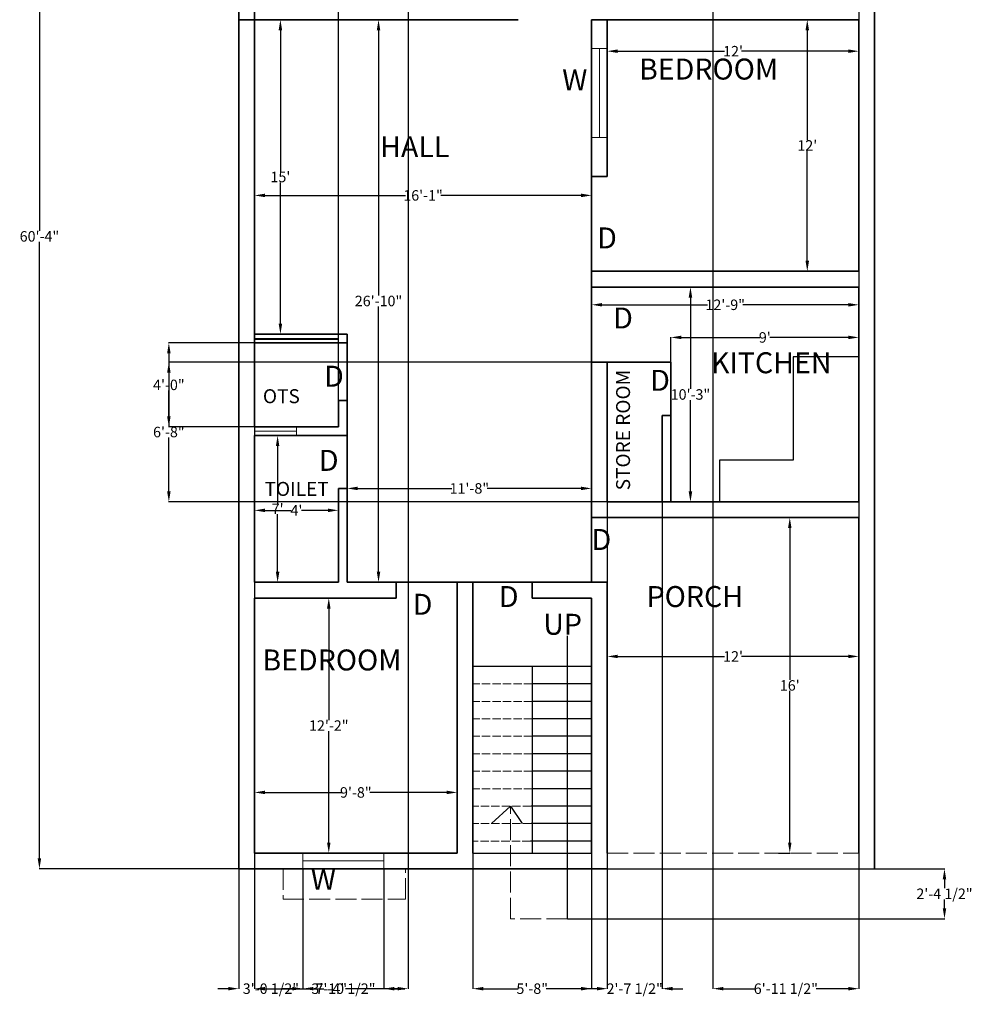
# Model space of a CAD drawing. Units: inches. Extents: x -732 to -187, y 754 to 1605.
# Tile 1 of 2: x -732 to -187, y 754 to 1318. Entities that reach past the tile are written whole.
import ezdxf

# ---------------------------------------------------------------- set-up
doc = ezdxf.new("R2010")
doc.units = ezdxf.units.IN
doc.header["$MEASUREMENT"] = 0
doc.linetypes.add('ACAD_ISO02W100', pattern=[15, 12, -3])
for name, color, linetype, lineweight in [('A-ANNO-DIMS', 2, 'Continuous', 18), ('A-ANNO-TEXT', 3, 'Continuous', 18), ('A-AREA-IDEN', 7, 'Continuous', 25), ('A-FLOR-CASE', 8, 'Continuous', 25), ('A-FLOR-STRS', 3, 'Continuous', 25), ('A-FLOR-STRS-HIDN', 3, 'ACAD_ISO02W100', 18), ('A-GLAZ', 4, 'Continuous', 18), ('A-ROOF-OVHD', 8, 'ACAD_ISO02W100', 18), ('A-WALL', 7, 'Continuous', 35)]:
    doc.layers.add(name, color=color, linetype=linetype, lineweight=lineweight)
doc.styles.get("Standard").update_dxf_attribs({"font": 'arial.ttf'})
doc.dimstyles.get("Standard").update_dxf_attribs({"dimtxt": 6, "dimasz": 6, "dimexe": 0.18, "dimexo": 0.0625, "dimgap": 0.09, "dimtad": 0, "dimtih": 1, "dimtoh": 1, "dimdec": 0, "dimzin": 0, "dimdsep": 46, "dimlunit": 3, "dimtxsty": 'Standard', "dimcen": 0.09, "dimadec": 0, "dimazin": 0, "dimtfac": 1, "dimtdec": 0, "dimtofl": 0, "dimtmove": 0, "dimatfit": 3, "dimfxl": 1, "dimtolj": 1, "dimtzin": 0, "dimarcsym": 0})

# ---------------------------------------------------------------- blocks, each defined once
blk = doc.blocks.new('*D4')
at = {"layer": 'A-ANNO-DIMS', "color": 0, "lineweight": -2, "transparency": 16777216}
for p, q in [((-597.28, 886.17), (-597.28, 875.44)), ((-481.28, 886.17), (-481.28, 875.44)), ((-591.28, 875.62), (-547.34, 875.62)), ((-487.28, 875.62), (-531.21, 875.62))]:
    blk.add_line(p, q, dxfattribs=at)
at = {"layer": 'A-ANNO-DIMS', "color": 0, "transparency": 16777216}
for points in [[(-591.28, 876.62), (-591.28, 874.62), (-597.28, 875.62)], [(-487.28, 876.62), (-487.28, 874.62), (-481.28, 875.62)]]:
    blk.add_solid(points, dxfattribs=at)
at = {"layer": 'Defpoints', "color": 0, "transparency": 16777216}
for p in [(-597.28, 886.23), (-481.28, 886.23), (-481.28, 875.62)]:
    blk.add_point(p, dxfattribs=at)
at = {"layer": 'A-ANNO-DIMS', "color": 0, "transparency": 16777216, "insert": (-539.28, 875.62), "char_height": 6, "attachment_point": 5}
blk.add_mtext('\\A1;9\'-8"', dxfattribs=at)
blk = doc.blocks.new('*D5')
at = {"layer": 'A-ANNO-DIMS', "color": 0, "lineweight": -2, "transparency": 16777216}
for p, q in [((-544.34, 986.88), (-554.94, 986.88)), ((-554.76, 980.88), (-554.76, 916.98)), ((-554.76, 846.88), (-554.76, 910.77)), ((-544.34, 840.88), (-554.94, 840.88))]:
    blk.add_line(p, q, dxfattribs=at)
at = {"layer": 'A-ANNO-DIMS', "color": 0, "transparency": 16777216}
for points in [[(-555.76, 980.88), (-553.76, 980.88), (-554.76, 986.88)], [(-555.76, 846.88), (-553.76, 846.88), (-554.76, 840.88)]]:
    blk.add_solid(points, dxfattribs=at)
at = {"layer": 'Defpoints', "color": 0, "transparency": 16777216}
for p in [(-544.28, 986.88), (-554.76, 840.88), (-544.28, 840.88)]:
    blk.add_point(p, dxfattribs=at)
at = {"layer": 'A-ANNO-DIMS', "color": 0, "transparency": 16777216, "insert": (-554.76, 913.88), "char_height": 6, "attachment_point": 5}
blk.add_mtext('\\A1;12\'-2"', dxfattribs=at)
blk = doc.blocks.new('*D6')
at = {"layer": 'A-ANNO-DIMS', "color": 0, "lineweight": -2, "transparency": 16777216}
for p, q in [((-297.29, 1032.88), (-290.63, 1032.88)), ((-290.81, 1026.88), (-290.81, 940.03)), ((-290.81, 846.88), (-290.81, 933.72)), ((-297.29, 840.88), (-290.63, 840.88))]:
    blk.add_line(p, q, dxfattribs=at)
at = {"layer": 'A-ANNO-DIMS', "color": 0, "transparency": 16777216}
for points in [[(-291.81, 1026.88), (-289.81, 1026.88), (-290.81, 1032.88)], [(-291.81, 846.88), (-289.81, 846.88), (-290.81, 840.88)]]:
    blk.add_solid(points, dxfattribs=at)
at = {"layer": 'Defpoints', "color": 0, "transparency": 16777216}
for p in [(-297.35, 1032.88), (-297.35, 840.88), (-290.81, 840.88)]:
    blk.add_point(p, dxfattribs=at)
at = {"layer": 'A-ANNO-DIMS', "color": 0, "transparency": 16777216, "insert": (-290.81, 936.88), "char_height": 6, "attachment_point": 5}
blk.add_mtext("\\A1;16'", dxfattribs=at)
blk = doc.blocks.new('*D7')
at = {"layer": 'A-ANNO-DIMS', "color": 0, "lineweight": -2, "transparency": 16777216}
for p, q in [((-395.28, 939.28), (-395.28, 953.64)), ((-389.28, 953.46), (-328.18, 953.46)), ((-257.28, 953.46), (-318.38, 953.46)), ((-251.28, 939.28), (-251.28, 953.64))]:
    blk.add_line(p, q, dxfattribs=at)
at = {"layer": 'A-ANNO-DIMS', "color": 0, "transparency": 16777216}
for points in [[(-389.28, 954.46), (-389.28, 952.46), (-395.28, 953.46)], [(-257.28, 954.46), (-257.28, 952.46), (-251.28, 953.46)]]:
    blk.add_solid(points, dxfattribs=at)
at = {"layer": 'Defpoints', "color": 0, "transparency": 16777216}
for p in [(-251.28, 953.46), (-395.28, 939.22), (-251.28, 939.22)]:
    blk.add_point(p, dxfattribs=at)
at = {"layer": 'A-ANNO-DIMS', "color": 0, "transparency": 16777216, "insert": (-323.28, 953.46), "char_height": 6, "attachment_point": 5}
blk.add_mtext("\\A1;12'", dxfattribs=at)
blk = doc.blocks.new('*D8')
at = {"layer": 'A-ANNO-DIMS', "color": 0, "lineweight": -2, "transparency": 16777216}
for p, q in [((-597.28, 1037.81), (-597.28, 1036.88)), ((-591.28, 1037.06), (-576.25, 1037.06)), ((-555.28, 1037.06), (-570.31, 1037.06)), ((-549.28, 1037.81), (-549.28, 1036.88))]:
    blk.add_line(p, q, dxfattribs=at)
at = {"layer": 'A-ANNO-DIMS', "color": 0, "transparency": 16777216}
for points in [[(-591.28, 1038.06), (-591.28, 1036.06), (-597.28, 1037.06)], [(-555.28, 1038.06), (-555.28, 1036.06), (-549.28, 1037.06)]]:
    blk.add_solid(points, dxfattribs=at)
at = {"layer": 'Defpoints', "color": 0, "transparency": 16777216}
for p in [(-597.28, 1037.88), (-549.28, 1037.88), (-549.28, 1037.06)]:
    blk.add_point(p, dxfattribs=at)
at = {"layer": 'A-ANNO-DIMS', "color": 0, "transparency": 16777216, "insert": (-573.28, 1037.06), "char_height": 6, "attachment_point": 5}
blk.add_mtext("\\A1;4'", dxfattribs=at)
blk = doc.blocks.new('*D9')
at = {"layer": 'A-ANNO-DIMS', "color": 0, "lineweight": -2, "transparency": 16777216}
for p, q in [((-587.22, 1079.88), (-583.88, 1079.88)), ((-584.06, 1073.88), (-584.06, 1040.97)), ((-584.06, 1001.88), (-584.06, 1034.79)), ((-587.22, 995.88), (-583.88, 995.88))]:
    blk.add_line(p, q, dxfattribs=at)
at = {"layer": 'A-ANNO-DIMS', "color": 0, "transparency": 16777216}
for points in [[(-585.06, 1073.88), (-583.06, 1073.88), (-584.06, 1079.88)], [(-585.06, 1001.88), (-583.06, 1001.88), (-584.06, 995.88)]]:
    blk.add_solid(points, dxfattribs=at)
at = {"layer": 'Defpoints', "color": 0, "transparency": 16777216}
for p in [(-587.28, 1079.88), (-587.28, 995.88), (-584.06, 995.88)]:
    blk.add_point(p, dxfattribs=at)
at = {"layer": 'A-ANNO-DIMS', "color": 0, "transparency": 16777216, "insert": (-584.06, 1037.88), "char_height": 6, "attachment_point": 5}
blk.add_mtext("\\A1;7'", dxfattribs=at)
blk = doc.blocks.new('*D10')
at = {"layer": 'A-ANNO-DIMS', "color": 0, "lineweight": -2, "transparency": 16777216}
for p, q in [((-544.28, 1049.68), (-544.28, 1049.8)), ((-538.28, 1049.62), (-484.39, 1049.62)), ((-410.28, 1049.62), (-464.17, 1049.62)), ((-404.28, 1049.68), (-404.28, 1049.8))]:
    blk.add_line(p, q, dxfattribs=at)
at = {"layer": 'A-ANNO-DIMS', "color": 0, "transparency": 16777216}
for points in [[(-538.28, 1050.62), (-538.28, 1048.62), (-544.28, 1049.62)], [(-410.28, 1050.62), (-410.28, 1048.62), (-404.28, 1049.62)]]:
    blk.add_solid(points, dxfattribs=at)
at = {"layer": 'Defpoints', "color": 0, "transparency": 16777216}
for p in [(-544.28, 1049.62), (-404.28, 1049.62), (-404.28, 1049.62)]:
    blk.add_point(p, dxfattribs=at)
at = {"layer": 'A-ANNO-DIMS', "color": 0, "transparency": 16777216, "insert": (-474.28, 1049.62), "char_height": 6, "attachment_point": 5}
blk.add_mtext('\\A1;11\'-8"', dxfattribs=at)
blk = doc.blocks.new('*D11')
at = {"layer": 'A-ANNO-DIMS', "color": 0, "lineweight": -2, "transparency": 16777216}
for p, q in [((-404.28, 1154.77), (-404.28, 1154.89)), ((-398.28, 1154.71), (-337.89, 1154.71)), ((-257.28, 1154.71), (-317.67, 1154.71)), ((-251.28, 1154.77), (-251.28, 1154.89))]:
    blk.add_line(p, q, dxfattribs=at)
at = {"layer": 'A-ANNO-DIMS', "color": 0, "transparency": 16777216}
for points in [[(-398.28, 1155.71), (-398.28, 1153.71), (-404.28, 1154.71)], [(-257.28, 1155.71), (-257.28, 1153.71), (-251.28, 1154.71)]]:
    blk.add_solid(points, dxfattribs=at)
at = {"layer": 'Defpoints', "color": 0, "transparency": 16777216}
for p in [(-404.28, 1154.71), (-251.28, 1154.71), (-251.28, 1154.71)]:
    blk.add_point(p, dxfattribs=at)
at = {"layer": 'A-ANNO-DIMS', "color": 0, "transparency": 16777216, "insert": (-327.78, 1154.71), "char_height": 6, "attachment_point": 5}
blk.add_mtext('\\A1;12\'-9"', dxfattribs=at)
blk = doc.blocks.new('*D12')
at = {"layer": 'A-ANNO-DIMS', "color": 0, "lineweight": -2, "transparency": 16777216}
for p, q in [((-347.74, 1164.88), (-347.86, 1164.88)), ((-347.68, 1158.88), (-347.68, 1106.53)), ((-347.68, 1047.88), (-347.68, 1100.22)), ((-347.74, 1041.88), (-347.86, 1041.88))]:
    blk.add_line(p, q, dxfattribs=at)
at = {"layer": 'A-ANNO-DIMS', "color": 0, "transparency": 16777216}
for points in [[(-348.68, 1158.88), (-346.68, 1158.88), (-347.68, 1164.88)], [(-348.68, 1047.88), (-346.68, 1047.88), (-347.68, 1041.88)]]:
    blk.add_solid(points, dxfattribs=at)
at = {"layer": 'Defpoints', "color": 0, "transparency": 16777216}
for p in [(-347.68, 1164.88), (-347.68, 1041.88), (-347.68, 1041.88)]:
    blk.add_point(p, dxfattribs=at)
at = {"layer": 'A-ANNO-DIMS', "color": 0, "transparency": 16777216, "insert": (-347.68, 1103.38), "char_height": 6, "attachment_point": 5}
blk.add_mtext('\\A1;10\'-3"', dxfattribs=at)
blk = doc.blocks.new('*D13')
at = {"layer": 'A-ANNO-DIMS', "color": 0, "lineweight": -2, "transparency": 16777216}
for p, q in [((-358.95, 1121.95), (-358.95, 1136.21)), ((-352.95, 1136.03), (-307.96, 1136.03)), ((-257.28, 1136.03), (-302.26, 1136.03)), ((-251.28, 1125.07), (-251.28, 1136.21))]:
    blk.add_line(p, q, dxfattribs=at)
at = {"layer": 'A-ANNO-DIMS', "color": 0, "transparency": 16777216}
for points in [[(-352.95, 1137.03), (-352.95, 1135.03), (-358.95, 1136.03)], [(-257.28, 1137.03), (-257.28, 1135.03), (-251.28, 1136.03)]]:
    blk.add_solid(points, dxfattribs=at)
at = {"layer": 'Defpoints', "color": 0, "transparency": 16777216}
for p in [(-251.28, 1136.03), (-358.95, 1121.89), (-251.28, 1125.01)]:
    blk.add_point(p, dxfattribs=at)
at = {"layer": 'A-ANNO-DIMS', "color": 0, "transparency": 16777216, "insert": (-305.11, 1136.03), "char_height": 6, "attachment_point": 5}
blk.add_mtext("\\A1;9'", dxfattribs=at)
blk = doc.blocks.new('*D14')
at = {"layer": 'A-ANNO-DIMS', "color": 0, "lineweight": -2, "transparency": 16777216}
for p, q in [((-585.31, 1317.88), (-582.28, 1317.88)), ((-582.46, 1311.88), (-582.46, 1231.03)), ((-582.46, 1143.88), (-582.46, 1224.72)), ((-585.31, 1137.88), (-582.28, 1137.88))]:
    blk.add_line(p, q, dxfattribs=at)
at = {"layer": 'A-ANNO-DIMS', "color": 0, "transparency": 16777216}
for points in [[(-583.46, 1311.88), (-581.46, 1311.88), (-582.46, 1317.88)], [(-583.46, 1143.88), (-581.46, 1143.88), (-582.46, 1137.88)]]:
    blk.add_solid(points, dxfattribs=at)
at = {"layer": 'Defpoints', "color": 0, "transparency": 16777216}
for p in [(-585.37, 1317.88), (-585.37, 1137.88), (-582.46, 1137.88)]:
    blk.add_point(p, dxfattribs=at)
at = {"layer": 'A-ANNO-DIMS', "color": 0, "transparency": 16777216, "insert": (-582.46, 1227.88), "char_height": 6, "attachment_point": 5}
blk.add_mtext("\\A1;15'", dxfattribs=at)
blk = doc.blocks.new('*D15')
at = {"layer": 'A-ANNO-DIMS', "color": 0, "lineweight": -2, "transparency": 16777216}
for p, q in [((-251.34, 1317.88), (-280.96, 1317.88)), ((-280.78, 1311.88), (-280.78, 1248.98)), ((-280.78, 1179.88), (-280.78, 1242.77)), ((-251.34, 1173.88), (-280.96, 1173.88))]:
    blk.add_line(p, q, dxfattribs=at)
at = {"layer": 'A-ANNO-DIMS', "color": 0, "transparency": 16777216}
for points in [[(-281.78, 1311.88), (-279.78, 1311.88), (-280.78, 1317.88)], [(-281.78, 1179.88), (-279.78, 1179.88), (-280.78, 1173.88)]]:
    blk.add_solid(points, dxfattribs=at)
at = {"layer": 'Defpoints', "color": 0, "transparency": 16777216}
for p in [(-251.28, 1317.88), (-280.78, 1173.88), (-251.28, 1173.88)]:
    blk.add_point(p, dxfattribs=at)
at = {"layer": 'A-ANNO-DIMS', "color": 0, "transparency": 16777216, "insert": (-280.78, 1245.88), "char_height": 6, "attachment_point": 5}
blk.add_mtext("\\A1;12'", dxfattribs=at)
blk = doc.blocks.new('*D16')
at = {"layer": 'A-ANNO-DIMS', "color": 0, "lineweight": -2, "transparency": 16777216}
for p, q in [((-395.28, 1317.81), (-395.28, 1299.67)), ((-251.28, 1317.81), (-251.28, 1299.67)), ((-389.28, 1299.85), (-328.18, 1299.85)), ((-257.28, 1299.85), (-318.38, 1299.85))]:
    blk.add_line(p, q, dxfattribs=at)
at = {"layer": 'A-ANNO-DIMS', "color": 0, "transparency": 16777216}
for points in [[(-389.28, 1300.85), (-389.28, 1298.85), (-395.28, 1299.85)], [(-257.28, 1300.85), (-257.28, 1298.85), (-251.28, 1299.85)]]:
    blk.add_solid(points, dxfattribs=at)
at = {"layer": 'Defpoints', "color": 0, "transparency": 16777216}
for p in [(-395.28, 1317.88), (-251.28, 1317.88), (-251.28, 1299.85)]:
    blk.add_point(p, dxfattribs=at)
at = {"layer": 'A-ANNO-DIMS', "color": 0, "transparency": 16777216, "insert": (-323.28, 1299.85), "char_height": 6, "attachment_point": 5}
blk.add_mtext("\\A1;12'", dxfattribs=at)
blk = doc.blocks.new('*D17')
at = {"layer": 'A-ANNO-DIMS', "color": 0, "lineweight": -2, "transparency": 16777216}
for p, q in [((-597.28, 1216.96), (-597.28, 1217.5)), ((-591.28, 1217.32), (-510.89, 1217.32)), ((-410.28, 1217.32), (-490.67, 1217.32)), ((-404.28, 1216.96), (-404.28, 1217.5))]:
    blk.add_line(p, q, dxfattribs=at)
at = {"layer": 'A-ANNO-DIMS', "color": 0, "transparency": 16777216}
for points in [[(-591.28, 1218.32), (-591.28, 1216.32), (-597.28, 1217.32)], [(-410.28, 1218.32), (-410.28, 1216.32), (-404.28, 1217.32)]]:
    blk.add_solid(points, dxfattribs=at)
at = {"layer": 'Defpoints', "color": 0, "transparency": 16777216}
for p in [(-404.28, 1217.32), (-597.28, 1216.9), (-404.28, 1216.9)]:
    blk.add_point(p, dxfattribs=at)
at = {"layer": 'A-ANNO-DIMS', "color": 0, "transparency": 16777216, "insert": (-500.78, 1217.32), "char_height": 6, "attachment_point": 5}
blk.add_mtext('\\A1;16\'-1"', dxfattribs=at)
blk = doc.blocks.new('*D18')
at = {"layer": 'A-ANNO-DIMS', "color": 0, "lineweight": -2, "transparency": 16777216}
for p, q in [((-526.34, 1317.88), (-526.46, 1317.88)), ((-526.28, 1311.88), (-526.28, 1160.03)), ((-526.28, 1001.88), (-526.28, 1153.72)), ((-526.34, 995.88), (-526.46, 995.88))]:
    blk.add_line(p, q, dxfattribs=at)
at = {"layer": 'A-ANNO-DIMS', "color": 0, "transparency": 16777216}
for points in [[(-527.28, 1311.88), (-525.28, 1311.88), (-526.28, 1317.88)], [(-527.28, 1001.88), (-525.28, 1001.88), (-526.28, 995.88)]]:
    blk.add_solid(points, dxfattribs=at)
at = {"layer": 'Defpoints', "color": 0, "transparency": 16777216}
for p in [(-526.28, 1317.88), (-526.28, 995.88), (-526.28, 995.88)]:
    blk.add_point(p, dxfattribs=at)
at = {"layer": 'A-ANNO-DIMS', "color": 0, "transparency": 16777216, "insert": (-526.28, 1156.88), "char_height": 6, "attachment_point": 5}
blk.add_mtext('\\A1;26\'-10"', dxfattribs=at)
blk = doc.blocks.new('*D24')
at = {"layer": 'A-ANNO-DIMS', "color": 0, "lineweight": -2, "transparency": 16777216}
for p, q in [((-606.34, 1555.88), (-720.61, 1555.88)), ((-720.43, 1549.88), (-720.43, 1197.03)), ((-720.43, 837.88), (-720.43, 1190.72)), ((-606.34, 831.88), (-720.61, 831.88))]:
    blk.add_line(p, q, dxfattribs=at)
at = {"layer": 'A-ANNO-DIMS', "color": 0, "transparency": 16777216}
for points in [[(-721.43, 1549.88), (-719.43, 1549.88), (-720.43, 1555.88)], [(-721.43, 837.88), (-719.43, 837.88), (-720.43, 831.88)]]:
    blk.add_solid(points, dxfattribs=at)
at = {"layer": 'Defpoints', "color": 0, "transparency": 16777216}
for p in [(-606.28, 1555.88), (-720.43, 831.88), (-606.28, 831.88)]:
    blk.add_point(p, dxfattribs=at)
at = {"layer": 'A-ANNO-DIMS', "color": 0, "transparency": 16777216, "insert": (-720.43, 1193.88), "char_height": 6, "attachment_point": 5}
blk.add_mtext('\\A1;60\'-4"', dxfattribs=at)
blk = doc.blocks.new('*D28')
at = {"layer": 'A-ANNO-DIMS', "color": 0, "lineweight": -2, "transparency": 16777216}
for p, q in [((-472.28, 840.81), (-472.28, 763.13)), ((-404.28, 840.81), (-404.28, 763.13)), ((-466.28, 763.31), (-446.34, 763.31)), ((-410.28, 763.31), (-430.21, 763.31))]:
    blk.add_line(p, q, dxfattribs=at)
at = {"layer": 'A-ANNO-DIMS', "color": 0, "transparency": 16777216}
for points in [[(-466.28, 764.31), (-466.28, 762.31), (-472.28, 763.31)], [(-410.28, 764.31), (-410.28, 762.31), (-404.28, 763.31)]]:
    blk.add_solid(points, dxfattribs=at)
at = {"layer": 'Defpoints', "color": 0, "transparency": 16777216}
for p in [(-472.28, 840.88), (-404.28, 840.88), (-404.28, 763.31)]:
    blk.add_point(p, dxfattribs=at)
at = {"layer": 'A-ANNO-DIMS', "color": 0, "transparency": 16777216, "insert": (-438.28, 763.31), "char_height": 6, "attachment_point": 5}
blk.add_mtext('\\A1;5\'-8"', dxfattribs=at)
blk = doc.blocks.new('*D29')
at = {"layer": 'A-ANNO-DIMS', "color": 0, "lineweight": -2, "transparency": 16777216}
for p, q in [((-395.22, 831.88), (-202.05, 831.88)), ((-202.23, 825.88), (-202.23, 820.81)), ((-202.23, 809.36), (-202.23, 814.42)), ((-418.12, 803.36), (-202.05, 803.36))]:
    blk.add_line(p, q, dxfattribs=at)
at = {"layer": 'A-ANNO-DIMS', "color": 0, "transparency": 16777216}
for points in [[(-203.23, 825.88), (-201.23, 825.88), (-202.23, 831.88)], [(-203.23, 809.36), (-201.23, 809.36), (-202.23, 803.36)]]:
    blk.add_solid(points, dxfattribs=at)
at = {"layer": 'Defpoints', "color": 0, "transparency": 16777216}
for p in [(-395.28, 831.88), (-418.19, 803.36), (-202.23, 803.36)]:
    blk.add_point(p, dxfattribs=at)
at = {"layer": 'A-ANNO-DIMS', "color": 0, "transparency": 16777216, "insert": (-202.23, 817.62), "char_height": 6, "attachment_point": 5}
blk.add_mtext('\\A1;2\'-4 1/2"', dxfattribs=at)
blk = doc.blocks.new('*D30')
at = {"layer": 'A-ANNO-DIMS', "color": 0, "lineweight": -2, "transparency": 16777216}
for p, q in [((-569.545923, 831.813688), (-569.545923, 763.128205)), ((-523.230383, 831.813688), (-523.230383, 763.128205)), ((-575.545923, 763.308205), (-581.545923, 763.308205)), ((-517.230383, 763.308205), (-511.230383, 763.308205))]:
    blk.add_line(p, q, dxfattribs=at)
at = {"layer": 'A-ANNO-DIMS', "color": 0, "transparency": 16777216}
for points in [[(-575.545923, 764.308205), (-575.545923, 762.308205), (-569.545923, 763.308205)], [(-517.230383, 764.308205), (-517.230383, 762.308205), (-523.230383, 763.308205)]]:
    blk.add_solid(points, dxfattribs=at)
at = {"layer": 'Defpoints', "color": 0, "transparency": 16777216}
for p in [(-569.545923, 831.876188), (-523.230383, 831.876188), (-523.230383, 763.308205)]:
    blk.add_point(p, dxfattribs=at)
at = {"layer": 'A-ANNO-DIMS', "color": 0, "transparency": 16777216, "insert": (-546.388153, 763.308205), "char_height": 6, "attachment_point": 5}
blk.add_mtext('\\A1;3\'-10 1/2"', dxfattribs=at)
blk = doc.blocks.new('*D31')
at = {"layer": 'A-ANNO-DIMS', "color": 0, "lineweight": -2, "transparency": 16777216}
for p, q in [((-606.28, 831.81), (-606.28, 763.13)), ((-569.55, 831.81), (-569.55, 763.13)), ((-612.28, 763.31), (-618.28, 763.31)), ((-563.55, 763.31), (-557.55, 763.31))]:
    blk.add_line(p, q, dxfattribs=at)
at = {"layer": 'A-ANNO-DIMS', "color": 0, "transparency": 16777216}
for points in [[(-612.28, 764.31), (-612.28, 762.31), (-606.28, 763.31)], [(-563.55, 764.31), (-563.55, 762.31), (-569.55, 763.31)]]:
    blk.add_solid(points, dxfattribs=at)
at = {"layer": 'Defpoints', "color": 0, "transparency": 16777216}
for p in [(-606.28, 831.88), (-569.55, 831.88), (-569.55, 763.31)]:
    blk.add_point(p, dxfattribs=at)
at = {"layer": 'A-ANNO-DIMS', "color": 0, "transparency": 16777216, "insert": (-587.91, 763.31), "char_height": 6, "attachment_point": 5}
blk.add_mtext('\\A1;3\'-0 1/2"', dxfattribs=at)
blk = doc.blocks.new('*D32')
at = {"layer": 'A-ANNO-DIMS', "color": 0, "lineweight": -2, "transparency": 16777216}
for p, q in [((-597.34, 1132.88), (-646.51, 1132.88)), ((-646.33, 1126.88), (-646.33, 1112.03)), ((-646.33, 1090.88), (-646.33, 1105.72)), ((-597.34, 1084.88), (-646.51, 1084.88))]:
    blk.add_line(p, q, dxfattribs=at)
at = {"layer": 'A-ANNO-DIMS', "color": 0, "transparency": 16777216}
for points in [[(-647.33, 1126.88), (-645.33, 1126.88), (-646.33, 1132.88)], [(-647.33, 1090.88), (-645.33, 1090.88), (-646.33, 1084.88)]]:
    blk.add_solid(points, dxfattribs=at)
at = {"layer": 'Defpoints', "color": 0, "transparency": 16777216}
for p in [(-646.33, 1132.88), (-597.28, 1132.88), (-597.28, 1084.88)]:
    blk.add_point(p, dxfattribs=at)
at = {"layer": 'A-ANNO-DIMS', "color": 0, "transparency": 16777216, "insert": (-646.33, 1108.88), "char_height": 6, "attachment_point": 5}
blk.add_mtext('\\A1;4\'-0"', dxfattribs=at)
blk = doc.blocks.new('*D33')
at = {"layer": 'A-ANNO-DIMS', "color": 0, "lineweight": -2, "transparency": 16777216}
for p, q in [((-597.28, 1084.94), (-597.28, 1596.11)), ((-591.28, 1595.93), (-581.46, 1595.93)), ((-555.28, 1595.93), (-565.09, 1595.93)), ((-549.28, 1084.94), (-549.28, 1596.11))]:
    blk.add_line(p, q, dxfattribs=at)
at = {"layer": 'A-ANNO-DIMS', "color": 0, "transparency": 16777216}
for points in [[(-591.28, 1596.93), (-591.28, 1594.93), (-597.28, 1595.93)], [(-555.28, 1596.93), (-555.28, 1594.93), (-549.28, 1595.93)]]:
    blk.add_solid(points, dxfattribs=at)
at = {"layer": 'Defpoints', "color": 0, "transparency": 16777216}
for p in [(-549.28, 1595.93), (-597.28, 1084.88), (-549.28, 1084.88)]:
    blk.add_point(p, dxfattribs=at)
at = {"layer": 'A-ANNO-DIMS', "color": 0, "transparency": 16777216, "insert": (-573.28, 1595.93), "char_height": 6, "attachment_point": 5}
blk.add_mtext('\\A1;4\'-0"', dxfattribs=at)
blk = doc.blocks.new('*D34')
at = {"layer": 'A-ANNO-DIMS', "color": 0, "lineweight": -2, "transparency": 16777216}
for p, q in [((-395.28, 1041.81), (-395.28, 763.13)), ((-363.95, 1041.81), (-363.95, 763.13)), ((-401.28, 763.31), (-407.28, 763.31)), ((-357.95, 763.31), (-351.95, 763.31))]:
    blk.add_line(p, q, dxfattribs=at)
at = {"layer": 'A-ANNO-DIMS', "color": 0, "transparency": 16777216}
for points in [[(-401.28, 764.31), (-401.28, 762.31), (-395.28, 763.31)], [(-357.95, 764.31), (-357.95, 762.31), (-363.95, 763.31)]]:
    blk.add_solid(points, dxfattribs=at)
at = {"layer": 'Defpoints', "color": 0, "transparency": 16777216}
for p in [(-395.28, 1041.88), (-363.95, 1041.88), (-363.95, 763.31)]:
    blk.add_point(p, dxfattribs=at)
at = {"layer": 'A-ANNO-DIMS', "color": 0, "transparency": 16777216, "insert": (-379.61, 763.31), "char_height": 6, "attachment_point": 5}
blk.add_mtext('\\A1;2\'-7 1/2"', dxfattribs=at)
blk = doc.blocks.new('*D35')
at = {"layer": 'A-ANNO-DIMS', "color": 0, "lineweight": -2, "transparency": 16777216}
for p, q in [((-395.34, 1121.89), (-646.51, 1121.89)), ((-646.33, 1115.89), (-646.33, 1085.04)), ((-646.33, 1047.88), (-646.33, 1078.73)), ((-395.34, 1041.88), (-646.51, 1041.88))]:
    blk.add_line(p, q, dxfattribs=at)
at = {"layer": 'A-ANNO-DIMS', "color": 0, "transparency": 16777216}
for points in [[(-647.33, 1115.89), (-645.33, 1115.89), (-646.33, 1121.89)], [(-647.33, 1047.88), (-645.33, 1047.88), (-646.33, 1041.88)]]:
    blk.add_solid(points, dxfattribs=at)
at = {"layer": 'Defpoints', "color": 0, "transparency": 16777216}
for p in [(-646.33, 1121.89), (-395.28, 1121.89), (-395.28, 1041.88)]:
    blk.add_point(p, dxfattribs=at)
at = {"layer": 'A-ANNO-DIMS', "color": 0, "transparency": 16777216, "insert": (-646.33, 1081.88), "char_height": 6, "attachment_point": 5}
blk.add_mtext('\\A1;6\'-8"', dxfattribs=at)
blk = doc.blocks.new('*D37')
at = {"layer": 'A-ANNO-DIMS', "color": 0, "lineweight": -2, "transparency": 16777216}
for p, q in [((-597.28, 1494.81), (-597.28, 763.13)), ((-509.33, 1494.81), (-509.33, 763.13)), ((-591.28, 763.31), (-561.35, 763.31)), ((-515.33, 763.31), (-545.27, 763.31))]:
    blk.add_line(p, q, dxfattribs=at)
at = {"layer": 'A-ANNO-DIMS', "color": 0, "transparency": 16777216}
for points in [[(-591.28, 764.31), (-591.28, 762.31), (-597.28, 763.31)], [(-515.33, 764.31), (-515.33, 762.31), (-509.33, 763.31)]]:
    blk.add_solid(points, dxfattribs=at)
at = {"layer": 'Defpoints', "color": 0, "transparency": 16777216}
for p in [(-597.28, 1494.88), (-509.33, 1494.88), (-509.33, 763.31)]:
    blk.add_point(p, dxfattribs=at)
at = {"layer": 'A-ANNO-DIMS', "color": 0, "transparency": 16777216, "insert": (-553.31, 763.31), "char_height": 6, "attachment_point": 5}
blk.add_mtext('\\A1;7\'-4"', dxfattribs=at)
blk = doc.blocks.new('*D38')
at = {"layer": 'A-ANNO-DIMS', "color": 0, "lineweight": -2, "transparency": 16777216}
for p, q in [((-334.82, 1494.81), (-334.82, 763.13)), ((-251.28, 1494.82), (-251.28, 763.13)), ((-328.82, 763.31), (-310.45, 763.31)), ((-257.28, 763.31), (-275.65, 763.31))]:
    blk.add_line(p, q, dxfattribs=at)
at = {"layer": 'A-ANNO-DIMS', "color": 0, "transparency": 16777216}
for points in [[(-328.82, 764.31), (-328.82, 762.31), (-334.82, 763.31)], [(-257.28, 764.31), (-257.28, 762.31), (-251.28, 763.31)]]:
    blk.add_solid(points, dxfattribs=at)
at = {"layer": 'Defpoints', "color": 0, "transparency": 16777216}
for p in [(-334.82, 1494.88), (-251.28, 1494.88), (-251.28, 763.31)]:
    blk.add_point(p, dxfattribs=at)
at = {"layer": 'A-ANNO-DIMS', "color": 0, "transparency": 16777216, "insert": (-293.05, 763.31), "char_height": 6, "attachment_point": 5}
blk.add_mtext('\\A1;6\'-11 1/2"', dxfattribs=at)

msp = doc.modelspace()

# ---------------------------------------------------------------- linework, layer by layer
at = {"layer": 'A-FLOR-CASE'}
for p, q in [((-251.28, 1125.01), (-288.91, 1125.01)), ((-288.91, 1125.01), (-288.91, 1065.83)), ((-288.91, 1065.83), (-331.08, 1065.83)), ((-331.08, 1065.83), (-331.08, 1041.88))]:
    msp.add_line(p, q, dxfattribs=at)
at = {"layer": 'A-FLOR-STRS'}
for p, q in [((-418.19, 965.32), (-418.19, 803.36)), ((-438.28, 947.75), (-472.28, 947.75)), ((-404.28, 947.75), (-438.28, 947.75)), ((-438.28, 947.75), (-438.28, 840.88)), ((-404.28, 937.75), (-438.28, 937.75)), ((-404.28, 927.75), (-438.28, 927.75)), ((-404.28, 917.75), (-438.28, 917.75)), ((-404.28, 907.75), (-438.28, 907.75)), ((-404.28, 897.75), (-438.28, 897.75)), ((-404.28, 887.75), (-438.28, 887.75)), ((-404.28, 877.75), (-438.28, 877.75)), ((-450.72, 867.75), (-461.68, 857.75)), ((-461.68, 857.75), (-450.72, 867.75)), ((-450.72, 867.75), (-444.04, 857.75)), ((-404.28, 867.75), (-438.93, 867.75)), ((-404.28, 857.75), (-438.93, 857.75)), ((-404.28, 847.75), (-439.17, 847.75)), ((-472.28, 840.88), (-404.28, 840.88))]:
    msp.add_line(p, q, dxfattribs=at)
at = {"layer": 'A-FLOR-STRS-HIDN', "ltscale": 0.4}
for p, q in [((-438.28, 937.75), (-472.28, 937.75)), ((-438.28, 927.75), (-472.28, 927.75)), ((-438.28, 917.75), (-472.28, 917.75)), ((-438.28, 907.75), (-472.28, 907.75)), ((-438.28, 897.75), (-472.28, 897.75)), ((-438.28, 887.75), (-472.28, 887.75)), ((-438.28, 877.75), (-472.28, 877.75)), ((-438.93, 867.75), (-472.28, 867.75)), ((-438.93, 857.75), (-472.28, 857.75)), ((-439.17, 847.75), (-472.28, 847.75))]:
    msp.add_line(p, q, dxfattribs=at)
at = {"layer": 'A-FLOR-STRS-HIDN'}
for p, q in [((-450.72, 803.36), (-450.72, 867.75)), ((-418.19, 803.36), (-450.72, 803.36))]:
    msp.add_line(p, q, dxfattribs=at)
at = {"layer": 'A-GLAZ'}
for p, q in [((-395.28, 1301.4), (-404.28, 1301.4)), ((-399.78, 1301.4), (-399.78, 1250.43)), ((-404.28, 1250.43), (-395.28, 1250.43)), ((-597.28, 1137.88), (-597.28, 1132.88)), ((-597.28, 1135.38), (-549.28, 1135.38)), ((-597.28, 1134.89), (-549.28, 1134.89)), ((-549.28, 1132.88), (-549.28, 1137.88)), ((-597.28, 1084.88), (-597.28, 1079.88)), ((-597.28, 1082.38), (-573.28, 1082.38)), ((-573.28, 1084.88), (-573.28, 1079.88)), ((-569.55, 840.88), (-569.55, 831.88)), ((-523.23, 840.88), (-523.23, 831.88)), ((-569.55, 836.38), (-523.23, 836.38))]:
    msp.add_line(p, q, dxfattribs=at)
at = {"layer": 'A-ROOF-OVHD'}
for p, q in [((-395.28, 840.88), (-251.28, 840.88)), ((-395.28, 840.88), (-395.28, 831.88)), ((-580.95, 831.88), (-580.95, 814.55)), ((-510.76, 814.55), (-510.76, 831.88)), ((-395.28, 831.88), (-242.28, 831.88)), ((-580.95, 814.55), (-510.76, 814.55))]:
    msp.add_line(p, q, dxfattribs=at)
at = {"layer": 'A-WALL'}
for p, q in [((-606.28, 1326.88), (-606.28, 831.88)), ((-242.28, 1326.88), (-242.28, 831.88)), ((-446.28, 1317.88), (-606.28, 1317.88)), ((-597.28, 1317.88), (-597.28, 1137.88)), ((-251.28, 1317.88), (-404.28, 1317.88)), ((-404.28, 1317.88), (-404.28, 1032.88)), ((-395.28, 1317.88), (-395.28, 1228.05)), ((-251.28, 1317.88), (-251.28, 1173.88)), ((-404.28, 1228.05), (-395.28, 1228.05)), ((-251.28, 1173.88), (-404.28, 1173.88)), ((-251.28, 1164.88), (-404.28, 1164.88)), ((-251.28, 1164.88), (-251.28, 1041.88)), ((-544.28, 1137.88), (-597.28, 1137.88)), ((-544.28, 1132.88), (-597.28, 1132.88)), ((-597.28, 1132.88), (-597.28, 1084.88)), ((-597.28, 1132.88), (-597.28, 1084.88)), ((-544.28, 1084.88), (-544.28, 1137.88)), ((-404.28, 1121.89), (-395.28, 1121.89)), ((-395.28, 1121.89), (-395.28, 1041.88)), ((-395.28, 1121.89), (-358.95, 1121.89)), ((-358.95, 1121.89), (-358.95, 1041.88)), ((-549.28, 1084.88), (-549.28, 1099.96)), ((-544.28, 1099.96), (-549.28, 1099.96)), ((-363.95, 1091.39), (-358.95, 1091.39)), ((-363.95, 1091.39), (-363.95, 1041.88)), ((-549.28, 1084.88), (-597.28, 1084.88)), ((-597.28, 1084.88), (-549.28, 1084.88)), ((-544.28, 995.88), (-544.28, 1084.88)), ((-549.28, 1079.88), (-597.28, 1079.88)), ((-597.28, 1079.88), (-597.28, 995.88)), ((-597.28, 1079.88), (-597.28, 995.88)), ((-549.28, 1079.88), (-544.28, 1079.88)), ((-549.28, 995.88), (-549.28, 1049.62)), ((-549.28, 1049.62), (-544.28, 1049.62)), ((-251.28, 1041.88), (-395.28, 1041.88)), ((-251.28, 1032.88), (-404.28, 1032.88)), ((-404.28, 1032.88), (-404.28, 995.88)), ((-251.28, 1032.88), (-395.28, 1032.88)), ((-251.28, 1032.88), (-251.28, 840.88)), ((-251.28, 840.88), (-251.28, 1032.88)), ((-597.28, 995.88), (-549.28, 995.88)), ((-549.28, 995.88), (-597.28, 995.88)), ((-395.28, 995.88), (-544.28, 995.88)), ((-516.26, 995.88), (-516.26, 986.88)), ((-481.28, 840.88), (-481.28, 995.88)), ((-472.28, 840.88), (-472.28, 995.88)), ((-438.28, 986.88), (-438.28, 995.88)), ((-395.28, 995.88), (-395.28, 840.88)), ((-597.28, 986.88), (-597.28, 840.88)), ((-597.28, 986.88), (-597.28, 840.88)), ((-516.26, 986.88), (-597.28, 986.88)), ((-404.28, 986.88), (-438.28, 986.88)), ((-404.28, 986.88), (-404.28, 840.88)), ((-597.28, 840.88), (-481.28, 840.88)), ((-597.28, 840.88), (-481.28, 840.88)), ((-606.28, 831.88), (-395.28, 831.88))]:
    msp.add_line(p, q, dxfattribs=at)

# ---------------------------------------------------------------- texts
at = {"layer": 'A-ANNO-TEXT', "char_height": 12, "attachment_point": 1}
for s, width, insert in [('W', 31.9676, (-421.1, 1289.42)), ('D', 8.414, (-401.08, 1198.97)), ('D', 8.414, (-391.89, 1153.15)), ('D', 8.414, (-557.43, 1119.84)), ('D', 8.414, (-370.7, 1117.47)), ('D', 8.414, (-560.4, 1071.66)), ('D', 8.414, (-404.28, 1026.38)), ('D', 8.414, (-457.35, 993.73)), ('D', 8.414, (-506.69, 989.29)), ('UP', 24.0231, (-431.93, 977.85)), ('W', 31.9676, (-565.05, 831.88))]:
    msp.add_mtext_dynamic_manual_height_columns(s, width=width, gutter_width=1, heights=[0], dxfattribs=dict(at, insert=insert))
at = {"layer": 'A-AREA-IDEN', "attachment_point": 1}
for s, width, insert, char_height in [('BEDROOM', 76.222, (-377.12, 1295.62), 12), ('HALL', 55.0492, (-525.33, 1251.21), 12), ('KITCHEN', 25.7938, (-335.92, 1127.53), 12), ('OTS', 13.784, (-592.48, 1106.4), 8), ('TOILET', 13.784, (-591.52, 1053.34), 8), ('PORCH', 90.4967, (-372.81, 993.73), 12), ('\\pxt8;BEDROOM', 71.5441, (-592.79, 957.43), 12)]:
    msp.add_mtext_dynamic_manual_height_columns(s, width=width, gutter_width=1, heights=[0], dxfattribs=dict(at, insert=insert, char_height=char_height))
at = {"layer": 'A-AREA-IDEN', "insert": (-390.26, 1048.52), "char_height": 8, "attachment_point": 1, "rotation": 90}
msp.add_mtext_dynamic_manual_height_columns('STORE ROOM', width=80.452, gutter_width=1, heights=[0], dxfattribs=at)

# ---------------------------------------------------------------- dimensions: what is measured, and where the dimension line sits
at = {"layer": 'A-ANNO-DIMS'}
for base, p1, p2, override, picture, middle in [((-549.28, 1595.93), (-597.28, 1084.88), (-549.28, 1084.88), {"dimdec": 1, "dimlfac": 1, "dimrnd": 0, "dimzin": 1, "dimdsep": 46, "dimlunit": 4, "dimfrac": 2}, '*D33', (-573.28, 1595.93)), ((-509.3331, 763.3082), (-597.2785, 1494.8762), (-509.3331, 1494.8762), {"dimdec": 1, "dimlfac": 1, "dimrnd": 0, "dimzin": 1, "dimdsep": 46, "dimlunit": 4, "dimfrac": 2}, '*D37', (-553.3058, 763.3082)), ((-251.28, 763.31), (-334.82, 1494.88), (-251.28, 1494.88), {"dimdec": 1, "dimlfac": 1, "dimrnd": 0, "dimzin": 1, "dimdsep": 46, "dimlunit": 4, "dimfrac": 2}, '*D38', (-293.05, 763.31)), ((-251.28, 1299.85), (-395.28, 1317.88), (-251.28, 1317.88), {"dimclrd": 0, "dimclre": 0, "dimclrt": 0}, '*D16', (-323.28, 1299.85)), ((-404.28, 1217.32), (-597.28, 1216.9), (-404.28, 1216.9), {"dimclrd": 0, "dimclre": 0, "dimclrt": 0}, '*D17', (-500.78, 1217.32)), ((-251.28, 1154.71), (-404.28, 1154.71), (-251.28, 1154.71), {"dimclrd": 0, "dimclre": 0, "dimclrt": 0}, '*D11', (-327.78, 1154.71)), ((-251.28, 1136.03), (-358.95, 1121.89), (-251.28, 1125.01), {"dimclrd": 0, "dimclre": 0, "dimclrt": 0}, '*D13', (-305.11, 1136.03)), ((-404.28, 1049.62), (-544.28, 1049.62), (-404.28, 1049.62), {"dimclrd": 0, "dimclre": 0, "dimclrt": 0}, '*D10', (-474.28, 1049.62)), ((-549.28, 1037.06), (-597.28, 1037.88), (-549.28, 1037.88), {"dimclrd": 0, "dimclre": 0, "dimclrt": 0}, '*D8', (-573.28, 1037.06)), ((-363.95, 763.31), (-395.28, 1041.88), (-363.95, 1041.88), {"dimdec": 1, "dimlfac": 1, "dimrnd": 0, "dimzin": 1, "dimdsep": 46, "dimlunit": 4, "dimfrac": 2}, '*D34', (-379.61, 763.31)), ((-251.28, 953.46), (-395.28, 939.22), (-251.28, 939.22), {"dimclrd": 0, "dimclre": 0, "dimclrt": 0}, '*D7', (-323.28, 953.46)), ((-481.28, 875.62), (-597.28, 886.23), (-481.28, 886.23), {"dimclrd": 0, "dimclre": 0, "dimclrt": 0}, '*D4', (-539.28, 875.62)), ((-404.28, 763.31), (-472.28, 840.88), (-404.28, 840.88), {"dimdec": 1, "dimlfac": 1, "dimrnd": 0, "dimzin": 1, "dimdsep": 46, "dimlunit": 4, "dimfrac": 2}, '*D28', (-438.28, 763.31)), ((-569.55, 763.31), (-606.28, 831.88), (-569.55, 831.88), {"dimdec": 1, "dimlfac": 1, "dimrnd": 0, "dimzin": 1, "dimdsep": 46, "dimlunit": 4, "dimfrac": 2}, '*D31', (-587.91, 763.31)), ((-523.23, 763.31), (-569.55, 831.88), (-523.23, 831.88), {"dimdec": 1, "dimlfac": 1, "dimrnd": 0, "dimzin": 1, "dimdsep": 46, "dimlunit": 4, "dimfrac": 2}, '*D30', (-546.39, 763.31))]:
    dim = msp.add_linear_dim(base=base, p1=p1, p2=p2, dimstyle='Standard', override=override, dxfattribs=at)
    dim.commit()
    dim.dimension.update_dxf_attribs({"geometry": picture, "text_midpoint": middle})
for base, p1, p2, override, picture, middle in [((-720.43, 831.88), (-606.28, 1555.88), (-606.28, 831.88), {"dimclrd": 0, "dimclre": 0, "dimclrt": 0}, '*D24', (-720.43, 1193.88)), ((-582.46, 1137.88), (-585.37, 1317.88), (-585.37, 1137.88), {"dimclrd": 0, "dimclre": 0, "dimclrt": 0}, '*D14', (-582.46, 1227.88)), ((-526.28, 995.88), (-526.28, 1317.88), (-526.28, 995.88), {"dimclrd": 0, "dimclre": 0, "dimclrt": 0}, '*D18', (-526.28, 1156.88)), ((-280.78, 1173.88), (-251.28, 1317.88), (-251.28, 1173.88), {"dimclrd": 0, "dimclre": 0, "dimclrt": 0}, '*D15', (-280.78, 1245.88)), ((-347.68, 1041.88), (-347.68, 1164.88), (-347.68, 1041.88), {"dimclrd": 0, "dimclre": 0, "dimclrt": 0}, '*D12', (-347.68, 1103.38)), ((-646.33, 1132.88), (-597.28, 1084.88), (-597.28, 1132.88), {"dimdec": 1, "dimlfac": 1, "dimrnd": 0, "dimzin": 1, "dimdsep": 46, "dimlunit": 4, "dimfrac": 2}, '*D32', (-646.33, 1108.88)), ((-646.33, 1121.89), (-395.28, 1041.88), (-395.28, 1121.89), {"dimdec": 1, "dimlfac": 1, "dimrnd": 0, "dimzin": 1, "dimdsep": 46, "dimlunit": 4, "dimfrac": 2}, '*D35', (-646.33, 1081.88)), ((-584.06, 995.88), (-587.28, 1079.88), (-587.28, 995.88), {"dimclrd": 0, "dimclre": 0, "dimclrt": 0}, '*D9', (-584.06, 1037.88)), ((-290.81, 840.88), (-297.35, 1032.88), (-297.35, 840.88), {"dimclrd": 0, "dimclre": 0, "dimclrt": 0}, '*D6', (-290.81, 936.88)), ((-554.76, 840.88), (-544.28, 986.88), (-544.28, 840.88), {"dimclrd": 0, "dimclre": 0, "dimclrt": 0}, '*D5', (-554.76, 913.88)), ((-202.23, 803.36), (-395.28, 831.88), (-418.19, 803.36), {"dimdec": 1, "dimlfac": 1, "dimrnd": 0, "dimzin": 1, "dimdsep": 46, "dimlunit": 4, "dimfrac": 2}, '*D29', (-202.23, 817.62))]:
    dim = msp.add_linear_dim(base=base, p1=p1, p2=p2, angle=90, dimstyle='Standard', override=override, dxfattribs=at)
    dim.commit()
    dim.dimension.update_dxf_attribs({"geometry": picture, "text_midpoint": middle})

doc.saveas('drawing.dxf')
